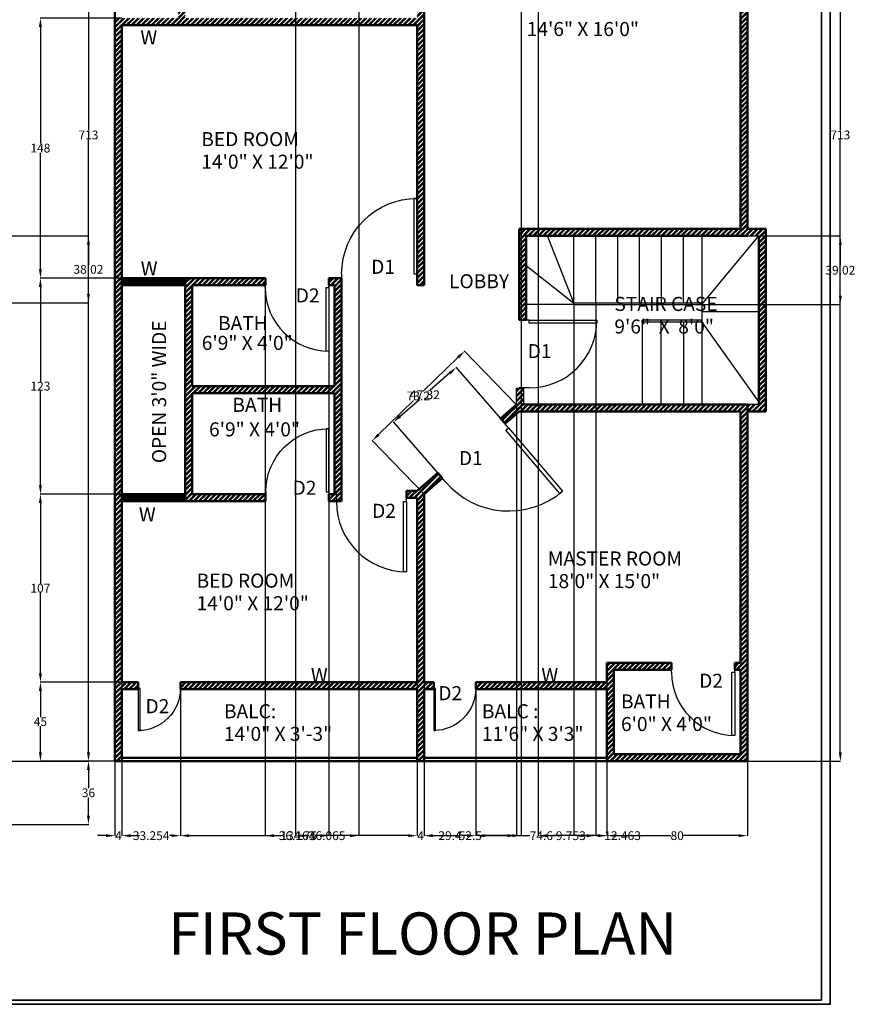
# Model space of a CAD drawing. Units: inches. Extents: x -35 to 905, y -602 to 298.
# Tile 3 of 4: x 429 to 905, y -602 to -42. Entities that reach past the tile are written whole.
import ezdxf

# ---------------------------------------------------------------- set-up
doc = ezdxf.new("R2010")
doc.units = ezdxf.units.IN
doc.header["$MEASUREMENT"] = 0
for name, color, linetype, lineweight in [('A-ANNO-DIMS', 2, 'Continuous', 18), ('A-ANNO-TEXT', 3, 'Continuous', 18), ('A-ANNO-TTLB', 7, 'Continuous', 35), ('A-AREA-IDEN', 7, 'Continuous', 18), ('A-COLS', 7, 'Continuous', 35), ('A-DOOR', 4, 'Continuous', 25), ('A-FLOR-STRS', 3, 'Continuous', 25), ('A-WALL', 7, 'Continuous', 50), ('A-WALL-PATT', 8, 'Continuous', 13)]:
    doc.layers.add(name, color=color, linetype=linetype, lineweight=lineweight)
doc.styles.get("Standard").update_dxf_attribs({"font": 'arial.ttf'})
doc.dimstyles.get("Standard").update_dxf_attribs({"dimtxt": 5, "dimasz": 5, "dimexe": 0.18, "dimexo": 0.0625, "dimgap": 0.09, "dimtad": 0, "dimtih": 1, "dimtoh": 1, "dimdec": 1, "dimzin": 0, "dimdsep": 46, "dimlunit": 4, "dimtxsty": 'Standard', "dimcen": 0.09, "dimadec": 0, "dimazin": 0, "dimtfac": 1, "dimtdec": 1, "dimtofl": 0, "dimtmove": 0, "dimatfit": 3, "dimfxl": 1, "dimtolj": 1, "dimtzin": 0, "dimarcsym": 0})

# ---------------------------------------------------------------- blocks, each defined once
blk = doc.blocks.new('*U2')
for p, q in [((0, 0), (0, -6)), ((40, 0), (40, -6))]:
    blk.add_line(p, q)
blk.add_lwpolyline([(0, 0), (0, 40), (1.75, 40), (1.75, 0)], close=True)
blk.add_arc((0, 0), 40, 0, 90)
blk = doc.blocks.new('*D17')
at = {"layer": 'A-ANNO-DIMS', "color": 0, "lineweight": -2, "ltscale": 0.3, "transparency": 16777216}
for p, q in [((377.85, -463.65), (468.36, -463.65)), ((468.18, -468.65), (468.18, -479.01)), ((468.18, -494.65), (468.18, -484.3)), ((377.85, -499.65), (468.36, -499.65))]:
    blk.add_line(p, q, dxfattribs=at)
at = {"layer": 'A-ANNO-DIMS', "color": 0, "ltscale": 0.3, "transparency": 16777216}
for points in [[(467.35, -468.65), (469.02, -468.65), (468.18, -463.65)], [(467.35, -494.65), (469.02, -494.65), (468.18, -499.65)]]:
    blk.add_solid(points, dxfattribs=at)
at = {"layer": 'Defpoints', "color": 0, "ltscale": 0.3, "transparency": 16777216}
for p in [(377.78, -463.65), (377.78, -499.65), (468.18, -499.65)]:
    blk.add_point(p, dxfattribs=at)
at = {"layer": 'A-ANNO-DIMS', "color": 0, "ltscale": 0.3, "transparency": 16777216, "insert": (468.18, -481.65), "char_height": 5, "attachment_point": 5}
blk.add_mtext('\\A1;36', dxfattribs=at)
blk = doc.blocks.new('*D18')
at = {"layer": 'A-ANNO-DIMS', "color": 0, "lineweight": -2, "ltscale": 0.3, "transparency": 16777216}
for p, q in [((377.85, 249.35), (468.36, 249.35)), ((468.18, 244.35), (468.18, -104.51)), ((468.18, -458.65), (468.18, -109.8)), ((377.85, -463.65), (468.36, -463.65))]:
    blk.add_line(p, q, dxfattribs=at)
at = {"layer": 'A-ANNO-DIMS', "color": 0, "ltscale": 0.3, "transparency": 16777216}
for points in [[(467.35, 244.35), (469.02, 244.35), (468.18, 249.35)], [(467.35, -458.65), (469.02, -458.65), (468.18, -463.65)]]:
    blk.add_solid(points, dxfattribs=at)
at = {"layer": 'Defpoints', "color": 0, "ltscale": 0.3, "transparency": 16777216}
for p in [(377.78, 249.35), (377.78, -463.65), (468.18, -463.65)]:
    blk.add_point(p, dxfattribs=at)
at = {"layer": 'A-ANNO-DIMS', "color": 0, "ltscale": 0.3, "transparency": 16777216, "insert": (468.18, -107.15), "char_height": 5, "attachment_point": 5}
blk.add_mtext('\\A1;713', dxfattribs=at)
blk = doc.blocks.new('*D28')
at = {"layer": 'A-ANNO-DIMS', "color": 0, "lineweight": -2, "ltscale": 0.3, "transparency": 16777216}
for p, q in [((279.1, -164.65), (468.36, -164.65)), ((468.18, -169.65), (468.18, -181.02)), ((468.18, -197.67), (468.18, -186.31)), ((279.1, -202.67), (468.36, -202.67))]:
    blk.add_line(p, q, dxfattribs=at)
at = {"layer": 'A-ANNO-DIMS', "color": 0, "ltscale": 0.3, "transparency": 16777216}
for points in [[(467.35, -169.65), (469.02, -169.65), (468.18, -164.65)], [(467.35, -197.67), (469.02, -197.67), (468.18, -202.67)]]:
    blk.add_solid(points, dxfattribs=at)
at = {"layer": 'Defpoints', "color": 0, "ltscale": 0.3, "transparency": 16777216}
for p in [(279.03, -164.65), (279.03, -202.67), (468.18, -202.67)]:
    blk.add_point(p, dxfattribs=at)
at = {"layer": 'A-ANNO-DIMS', "color": 0, "ltscale": 0.3, "transparency": 16777216, "insert": (468.18, -183.66), "char_height": 5, "attachment_point": 5}
blk.add_mtext('\\A1;38.02', dxfattribs=at)
blk = doc.blocks.new('*D36')
at = {"layer": 'A-ANNO-DIMS', "color": 0, "lineweight": -2, "ltscale": 0.3, "transparency": 16777216}
for p, q in [((487.18, -40.65), (440.66, -40.65)), ((440.84, -45.65), (440.84, -112.01)), ((440.84, -183.65), (440.84, -117.3)), ((487.18, -188.65), (440.66, -188.65))]:
    blk.add_line(p, q, dxfattribs=at)
at = {"layer": 'A-ANNO-DIMS', "color": 0, "ltscale": 0.3, "transparency": 16777216}
for points in [[(440.01, -45.65), (441.67, -45.65), (440.84, -40.65)], [(440.01, -183.65), (441.67, -183.65), (440.84, -188.65)]]:
    blk.add_solid(points, dxfattribs=at)
at = {"layer": 'Defpoints', "color": 0, "ltscale": 0.3, "transparency": 16777216}
for p in [(487.24, -40.65), (440.84, -188.65), (487.24, -188.65)]:
    blk.add_point(p, dxfattribs=at)
at = {"layer": 'A-ANNO-DIMS', "color": 0, "ltscale": 0.3, "transparency": 16777216, "insert": (440.84, -114.65), "char_height": 5, "attachment_point": 5}
blk.add_mtext('\\A1;148', dxfattribs=at)
blk = doc.blocks.new('*D37')
at = {"layer": 'A-ANNO-DIMS', "color": 0, "lineweight": -2, "ltscale": 0.3, "transparency": 16777216}
for p, q in [((487.18, -188.65), (440.66, -188.65)), ((440.84, -193.65), (440.84, -247.51)), ((440.84, -306.65), (440.84, -252.8)), ((487.18, -311.65), (440.66, -311.65))]:
    blk.add_line(p, q, dxfattribs=at)
at = {"layer": 'A-ANNO-DIMS', "color": 0, "ltscale": 0.3, "transparency": 16777216}
for points in [[(440.01, -193.65), (441.67, -193.65), (440.84, -188.65)], [(440.01, -306.65), (441.67, -306.65), (440.84, -311.65)]]:
    blk.add_solid(points, dxfattribs=at)
at = {"layer": 'Defpoints', "color": 0, "ltscale": 0.3, "transparency": 16777216}
for p in [(487.24, -188.65), (440.84, -311.65), (487.24, -311.65)]:
    blk.add_point(p, dxfattribs=at)
at = {"layer": 'A-ANNO-DIMS', "color": 0, "ltscale": 0.3, "transparency": 16777216, "insert": (440.84, -250.15), "char_height": 5, "attachment_point": 5}
blk.add_mtext('\\A1;123', dxfattribs=at)
blk = doc.blocks.new('*D38')
at = {"layer": 'A-ANNO-DIMS', "color": 0, "lineweight": -2, "ltscale": 0.3, "transparency": 16777216}
for p, q in [((487.18, -311.65), (440.66, -311.65)), ((440.84, -316.65), (440.84, -362.51)), ((440.84, -413.65), (440.84, -367.8)), ((487.18, -418.65), (440.66, -418.65))]:
    blk.add_line(p, q, dxfattribs=at)
at = {"layer": 'A-ANNO-DIMS', "color": 0, "ltscale": 0.3, "transparency": 16777216}
for points in [[(440.01, -316.65), (441.67, -316.65), (440.84, -311.65)], [(440.01, -413.65), (441.67, -413.65), (440.84, -418.65)]]:
    blk.add_solid(points, dxfattribs=at)
at = {"layer": 'Defpoints', "color": 0, "ltscale": 0.3, "transparency": 16777216}
for p in [(487.24, -311.65), (440.84, -418.65), (487.24, -418.65)]:
    blk.add_point(p, dxfattribs=at)
at = {"layer": 'A-ANNO-DIMS', "color": 0, "ltscale": 0.3, "transparency": 16777216, "insert": (440.84, -365.15), "char_height": 5, "attachment_point": 5}
blk.add_mtext('\\A1;107', dxfattribs=at)
blk = doc.blocks.new('*D39')
at = {"layer": 'A-ANNO-DIMS', "color": 0, "lineweight": -2, "ltscale": 0.3, "transparency": 16777216}
for p, q in [((487.18, -418.65), (440.66, -418.65)), ((440.84, -423.65), (440.84, -438.52)), ((440.84, -458.65), (440.84, -443.79)), ((483.18, -463.65), (440.66, -463.65))]:
    blk.add_line(p, q, dxfattribs=at)
at = {"layer": 'A-ANNO-DIMS', "color": 0, "ltscale": 0.3, "transparency": 16777216}
for points in [[(440.01, -423.65), (441.67, -423.65), (440.84, -418.65)], [(440.01, -458.65), (441.67, -458.65), (440.84, -463.65)]]:
    blk.add_solid(points, dxfattribs=at)
at = {"layer": 'Defpoints', "color": 0, "ltscale": 0.3, "transparency": 16777216}
for p in [(487.24, -418.65), (440.84, -463.65), (483.24, -463.65)]:
    blk.add_point(p, dxfattribs=at)
at = {"layer": 'A-ANNO-DIMS', "color": 0, "ltscale": 0.3, "transparency": 16777216, "insert": (440.84, -441.15), "char_height": 5, "attachment_point": 5}
blk.add_mtext('\\A1;45', dxfattribs=at)
blk = doc.blocks.new('*D40')
at = {"layer": 'A-ANNO-DIMS', "color": 0, "lineweight": -2, "ltscale": 0.3, "transparency": 16777216}
for p, q in [((843.3, 249.35), (896.28, 249.35)), ((896.1, 244.35), (896.1, -104.51)), ((896.1, -458.65), (896.1, -109.8)), ((843.3, -463.65), (896.28, -463.65))]:
    blk.add_line(p, q, dxfattribs=at)
at = {"layer": 'A-ANNO-DIMS', "color": 0, "ltscale": 0.3, "transparency": 16777216}
for points in [[(895.27, 244.35), (896.94, 244.35), (896.1, 249.35)], [(895.27, -458.65), (896.94, -458.65), (896.1, -463.65)]]:
    blk.add_solid(points, dxfattribs=at)
at = {"layer": 'Defpoints', "color": 0, "ltscale": 0.3, "transparency": 16777216}
for p in [(843.24, 249.35), (843.24, -463.65), (896.1, -463.65)]:
    blk.add_point(p, dxfattribs=at)
at = {"layer": 'A-ANNO-DIMS', "color": 0, "ltscale": 0.3, "transparency": 16777216, "insert": (896.1, -107.15), "char_height": 5, "attachment_point": 5}
blk.add_mtext('\\A1;713', dxfattribs=at)
blk = doc.blocks.new('*D41')
at = {"layer": 'A-ANNO-DIMS', "color": 0, "lineweight": -2, "ltscale": 0.3, "transparency": 16777216}
for p, q in [((487.24, -418.72), (487.24, -506.23)), ((483.24, -463.72), (483.24, -506.23)), ((478.24, -506.05), (473.24, -506.05)), ((492.24, -506.05), (497.24, -506.05))]:
    blk.add_line(p, q, dxfattribs=at)
at = {"layer": 'A-ANNO-DIMS', "color": 0, "ltscale": 0.3, "transparency": 16777216}
for points in [[(478.24, -505.22), (478.24, -506.89), (483.24, -506.05)], [(492.24, -505.22), (492.24, -506.89), (487.24, -506.05)]]:
    blk.add_solid(points, dxfattribs=at)
at = {"layer": 'Defpoints', "color": 0, "ltscale": 0.3, "transparency": 16777216}
for p in [(487.24, -418.65), (483.24, -463.65), (487.24, -506.05)]:
    blk.add_point(p, dxfattribs=at)
at = {"layer": 'A-ANNO-DIMS', "color": 0, "ltscale": 0.3, "transparency": 16777216, "insert": (485.24, -506.05), "char_height": 5, "attachment_point": 5}
blk.add_mtext('\\A1;4', dxfattribs=at)
blk = doc.blocks.new('*D42')
at = {"layer": 'A-ANNO-DIMS', "color": 0, "lineweight": -2, "ltscale": 0.3, "transparency": 16777216}
for p, q in [((487.24, -418.72), (487.24, -506.23)), ((520.49, -418.72), (520.49, -506.23)), ((492.24, -506.05), (493.41, -506.05)), ((515.49, -506.05), (514.32, -506.05))]:
    blk.add_line(p, q, dxfattribs=at)
at = {"layer": 'A-ANNO-DIMS', "color": 0, "ltscale": 0.3, "transparency": 16777216}
for points in [[(492.24, -505.22), (492.24, -506.89), (487.24, -506.05)], [(515.49, -505.22), (515.49, -506.89), (520.49, -506.05)]]:
    blk.add_solid(points, dxfattribs=at)
at = {"layer": 'Defpoints', "color": 0, "ltscale": 0.3, "transparency": 16777216}
for p in [(487.24, -418.65), (520.49, -418.65), (520.49, -506.05)]:
    blk.add_point(p, dxfattribs=at)
at = {"layer": 'A-ANNO-DIMS', "color": 0, "ltscale": 0.3, "transparency": 16777216, "insert": (503.87, -506.05), "char_height": 5, "attachment_point": 5}
blk.add_mtext('\\A1;33.254', dxfattribs=at)
blk = doc.blocks.new('*D43')
at = {"layer": 'A-ANNO-DIMS', "color": 0, "lineweight": -2, "ltscale": 0.3, "transparency": 16777216}
for p, q in [((520.49, -418.72), (520.49, -506.23)), ((655.24, -418.72), (655.24, -506.23)), ((525.49, -506.05), (577.61, -506.05)), ((650.24, -506.05), (598.12, -506.05))]:
    blk.add_line(p, q, dxfattribs=at)
at = {"layer": 'A-ANNO-DIMS', "color": 0, "ltscale": 0.3, "transparency": 16777216}
for points in [[(525.49, -505.22), (525.49, -506.89), (520.49, -506.05)], [(650.24, -505.22), (650.24, -506.89), (655.24, -506.05)]]:
    blk.add_solid(points, dxfattribs=at)
at = {"layer": 'Defpoints', "color": 0, "ltscale": 0.3, "transparency": 16777216}
for p in [(520.49, -418.65), (655.24, -418.65), (655.24, -506.05)]:
    blk.add_point(p, dxfattribs=at)
at = {"layer": 'A-ANNO-DIMS', "color": 0, "ltscale": 0.3, "transparency": 16777216, "insert": (587.87, -506.05), "char_height": 5, "attachment_point": 5}
blk.add_mtext('\\A1;134.75', dxfattribs=at)
blk = doc.blocks.new('*D44')
at = {"layer": 'A-ANNO-DIMS', "color": 0, "lineweight": -2, "ltscale": 0.3, "transparency": 16777216}
for p, q in [((655.24, -418.72), (655.24, -506.23)), ((659.24, -418.72), (659.24, -506.23)), ((650.24, -506.05), (645.24, -506.05)), ((664.24, -506.05), (669.24, -506.05))]:
    blk.add_line(p, q, dxfattribs=at)
at = {"layer": 'A-ANNO-DIMS', "color": 0, "ltscale": 0.3, "transparency": 16777216}
for points in [[(650.24, -505.22), (650.24, -506.89), (655.24, -506.05)], [(664.24, -505.22), (664.24, -506.89), (659.24, -506.05)]]:
    blk.add_solid(points, dxfattribs=at)
at = {"layer": 'Defpoints', "color": 0, "ltscale": 0.3, "transparency": 16777216}
for p in [(655.24, -418.65), (659.24, -418.65), (659.24, -506.05)]:
    blk.add_point(p, dxfattribs=at)
at = {"layer": 'A-ANNO-DIMS', "color": 0, "ltscale": 0.3, "transparency": 16777216, "insert": (657.24, -506.05), "char_height": 5, "attachment_point": 5}
blk.add_mtext('\\A1;4', dxfattribs=at)
blk = doc.blocks.new('*D45')
at = {"layer": 'A-ANNO-DIMS', "color": 0, "lineweight": -2, "ltscale": 0.3, "transparency": 16777216}
for p, q in [((659.24, -418.72), (659.24, -506.23)), ((688.64, -418.72), (688.64, -506.23)), ((664.24, -506.05), (667.32, -506.05)), ((683.64, -506.05), (680.55, -506.05))]:
    blk.add_line(p, q, dxfattribs=at)
at = {"layer": 'A-ANNO-DIMS', "color": 0, "ltscale": 0.3, "transparency": 16777216}
for points in [[(664.24, -505.22), (664.24, -506.89), (659.24, -506.05)], [(683.64, -505.22), (683.64, -506.89), (688.64, -506.05)]]:
    blk.add_solid(points, dxfattribs=at)
at = {"layer": 'Defpoints', "color": 0, "ltscale": 0.3, "transparency": 16777216}
for p in [(659.24, -418.65), (688.64, -418.65), (688.64, -506.05)]:
    blk.add_point(p, dxfattribs=at)
at = {"layer": 'A-ANNO-DIMS', "color": 0, "ltscale": 0.3, "transparency": 16777216, "insert": (673.94, -506.05), "char_height": 5, "attachment_point": 5}
blk.add_mtext('\\A1;29.4', dxfattribs=at)
blk = doc.blocks.new('*D46')
at = {"layer": 'A-ANNO-DIMS', "color": 0, "lineweight": -2, "ltscale": 0.3, "transparency": 16777216}
for p, q in [((688.64, -418.72), (688.64, -506.23)), ((763.24, -418.72), (763.24, -506.23)), ((693.64, -506.05), (719.38, -506.05)), ((758.24, -506.05), (732.5, -506.05))]:
    blk.add_line(p, q, dxfattribs=at)
at = {"layer": 'A-ANNO-DIMS', "color": 0, "ltscale": 0.3, "transparency": 16777216}
for points in [[(693.64, -505.22), (693.64, -506.89), (688.64, -506.05)], [(758.24, -505.22), (758.24, -506.89), (763.24, -506.05)]]:
    blk.add_solid(points, dxfattribs=at)
at = {"layer": 'Defpoints', "color": 0, "ltscale": 0.3, "transparency": 16777216}
for p in [(688.64, -418.65), (763.24, -418.65), (763.24, -506.05)]:
    blk.add_point(p, dxfattribs=at)
at = {"layer": 'A-ANNO-DIMS', "color": 0, "ltscale": 0.3, "transparency": 16777216, "insert": (725.94, -506.05), "char_height": 5, "attachment_point": 5}
blk.add_mtext('\\A1;74.6', dxfattribs=at)
blk = doc.blocks.new('*D47')
at = {"layer": 'A-ANNO-DIMS', "color": 0, "lineweight": -2, "ltscale": 0.3, "transparency": 16777216}
for p, q in [((763.24, -418.72), (763.24, -506.23)), ((843.24, -463.72), (843.24, -506.23)), ((768.24, -506.05), (799.57, -506.05)), ((838.24, -506.05), (806.9, -506.05))]:
    blk.add_line(p, q, dxfattribs=at)
at = {"layer": 'A-ANNO-DIMS', "color": 0, "ltscale": 0.3, "transparency": 16777216}
for points in [[(768.24, -505.22), (768.24, -506.89), (763.24, -506.05)], [(838.24, -505.22), (838.24, -506.89), (843.24, -506.05)]]:
    blk.add_solid(points, dxfattribs=at)
at = {"layer": 'Defpoints', "color": 0, "ltscale": 0.3, "transparency": 16777216}
for p in [(763.24, -418.65), (843.24, -463.65), (843.24, -506.05)]:
    blk.add_point(p, dxfattribs=at)
at = {"layer": 'A-ANNO-DIMS', "color": 0, "ltscale": 0.3, "transparency": 16777216, "insert": (803.24, -506.05), "char_height": 5, "attachment_point": 5}
blk.add_mtext('\\A1;80', dxfattribs=at)
blk = doc.blocks.new('*D48')
at = {"layer": 'A-ANNO-DIMS', "color": 0, "lineweight": -2, "ltscale": 0.3, "transparency": 16777216}
for p, q in [((585.99, 167.28), (585.99, -506.23)), ((622.06, 167.28), (622.06, -506.23)), ((590.99, -506.05), (593.54, -506.05)), ((617.06, -506.05), (614.51, -506.05))]:
    blk.add_line(p, q, dxfattribs=at)
at = {"layer": 'A-ANNO-DIMS', "color": 0, "ltscale": 0.3, "transparency": 16777216}
for points in [[(590.99, -505.22), (590.99, -506.89), (585.99, -506.05)], [(617.06, -505.22), (617.06, -506.89), (622.06, -506.05)]]:
    blk.add_solid(points, dxfattribs=at)
at = {"layer": 'Defpoints', "color": 0, "ltscale": 0.3, "transparency": 16777216}
for p in [(585.99, 167.35), (622.06, 167.35), (622.06, -506.05)]:
    blk.add_point(p, dxfattribs=at)
at = {"layer": 'A-ANNO-DIMS', "color": 0, "ltscale": 0.3, "transparency": 16777216, "insert": (604.02, -506.05), "char_height": 5, "attachment_point": 5}
blk.add_mtext('\\A1;36.065', dxfattribs=at)
blk = doc.blocks.new('*D49')
at = {"layer": 'A-ANNO-DIMS', "color": 0, "lineweight": -2, "ltscale": 0.3, "transparency": 16777216}
for p, q in [((568.83, -188.72), (568.83, -506.23)), ((604.99, -188.72), (604.99, -506.23)), ((573.83, -506.05), (576.45, -506.05)), ((599.99, -506.05), (597.37, -506.05))]:
    blk.add_line(p, q, dxfattribs=at)
at = {"layer": 'A-ANNO-DIMS', "color": 0, "ltscale": 0.3, "transparency": 16777216}
for points in [[(573.83, -505.22), (573.83, -506.89), (568.83, -506.05)], [(599.99, -505.22), (599.99, -506.89), (604.99, -506.05)]]:
    blk.add_solid(points, dxfattribs=at)
at = {"layer": 'Defpoints', "color": 0, "ltscale": 0.3, "transparency": 16777216}
for p in [(568.83, -188.65), (604.99, -188.65), (604.99, -506.05)]:
    blk.add_point(p, dxfattribs=at)
at = {"layer": 'A-ANNO-DIMS', "color": 0, "ltscale": 0.3, "transparency": 16777216, "insert": (586.91, -506.05), "char_height": 5, "attachment_point": 5}
blk.add_mtext('\\A1;36.164', dxfattribs=at)
blk = doc.blocks.new('*D50')
at = {"layer": 'A-ANNO-DIMS', "color": 0, "lineweight": -2, "ltscale": 0.3, "transparency": 16777216}
for p, q in [((705.33, -271.45), (677.42, -239.38)), ((673.76, -242.8), (662.73, -252.41)), ((645.62, -267.3), (656.65, -257.7)), ((669.64, -302.52), (641.73, -270.45))]:
    blk.add_line(p, q, dxfattribs=at)
at = {"layer": 'A-ANNO-DIMS', "color": 0, "ltscale": 0.3, "transparency": 16777216}
for points in [[(673.22, -242.17), (674.31, -243.43), (677.53, -239.52)], [(645.07, -266.67), (646.16, -267.93), (641.84, -270.58)]]:
    blk.add_solid(points, dxfattribs=at)
at = {"layer": 'Defpoints', "color": 0, "ltscale": 0.3, "transparency": 16777216}
for p in [(677.53, -239.52), (705.37, -271.5), (669.68, -302.57)]:
    blk.add_point(p, dxfattribs=at)
at = {"layer": 'A-ANNO-DIMS', "color": 0, "ltscale": 0.3, "transparency": 16777216, "insert": (659.69, -255.05), "char_height": 5, "attachment_point": 5}
blk.add_mtext('\\A1;47.32', dxfattribs=at)
blk = doc.blocks.new('*D52')
at = {"layer": 'A-ANNO-DIMS', "color": 0, "lineweight": -2, "ltscale": 0.3, "transparency": 16777216}
for p, q in [((714.42, 202.86), (714.42, -506.23)), ((724.17, 202.86), (724.17, -506.23)), ((709.42, -506.05), (704.42, -506.05)), ((729.17, -506.05), (734.17, -506.05))]:
    blk.add_line(p, q, dxfattribs=at)
at = {"layer": 'A-ANNO-DIMS', "color": 0, "ltscale": 0.3, "transparency": 16777216}
for points in [[(709.42, -505.22), (709.42, -506.89), (714.42, -506.05)], [(729.17, -505.22), (729.17, -506.89), (724.17, -506.05)]]:
    blk.add_solid(points, dxfattribs=at)
at = {"layer": 'Defpoints', "color": 0, "ltscale": 0.3, "transparency": 16777216}
for p in [(714.42, 202.92), (724.17, 202.92), (724.17, -506.05)]:
    blk.add_point(p, dxfattribs=at)
at = {"layer": 'A-ANNO-DIMS', "color": 0, "ltscale": 0.3, "transparency": 16777216, "insert": (742.7, -506.05), "char_height": 5, "attachment_point": 5}
blk.add_mtext('\\A1;9.753', dxfattribs=at)
blk = doc.blocks.new('*D54')
at = {"layer": 'A-ANNO-DIMS', "color": 0, "lineweight": -2, "ltscale": 0.3, "transparency": 16777216}
for p, q in [((744.49, -203.74), (744.49, -506.23)), ((756.95, -202.74), (756.95, -506.23)), ((749.49, -506.05), (751.95, -506.05)), ((756.95, -506.05), (761.95, -506.05))]:
    blk.add_line(p, q, dxfattribs=at)
at = {"layer": 'A-ANNO-DIMS', "color": 0, "ltscale": 0.3, "transparency": 16777216}
for points in [[(749.49, -505.22), (749.49, -506.89), (744.49, -506.05)], [(751.95, -505.22), (751.95, -506.89), (756.95, -506.05)]]:
    blk.add_solid(points, dxfattribs=at)
at = {"layer": 'Defpoints', "color": 0, "ltscale": 0.3, "transparency": 16777216}
for p in [(744.49, -203.67), (756.95, -202.67), (756.95, -506.05)]:
    blk.add_point(p, dxfattribs=at)
at = {"layer": 'A-ANNO-DIMS', "color": 0, "ltscale": 0.3, "transparency": 16777216, "insert": (772.18, -506.05), "char_height": 5, "attachment_point": 5}
blk.add_mtext('\\A1;12.463', dxfattribs=at)
blk = doc.blocks.new('*D55')
at = {"layer": 'A-ANNO-DIMS', "color": 0, "lineweight": -2, "ltscale": 0.3, "transparency": 16777216}
for p, q in [((744.55, -164.65), (896.28, -164.65)), ((896.1, -169.65), (896.1, -181.52)), ((896.1, -198.67), (896.1, -186.81)), ((744.55, -203.67), (896.28, -203.67))]:
    blk.add_line(p, q, dxfattribs=at)
at = {"layer": 'A-ANNO-DIMS', "color": 0, "ltscale": 0.3, "transparency": 16777216}
for points in [[(895.27, -169.65), (896.94, -169.65), (896.1, -164.65)], [(895.27, -198.67), (896.94, -198.67), (896.1, -203.67)]]:
    blk.add_solid(points, dxfattribs=at)
at = {"layer": 'Defpoints', "color": 0, "ltscale": 0.3, "transparency": 16777216}
for p in [(744.49, -164.65), (744.49, -203.67), (896.1, -203.67)]:
    blk.add_point(p, dxfattribs=at)
at = {"layer": 'A-ANNO-DIMS', "color": 0, "ltscale": 0.3, "transparency": 16777216, "insert": (896.1, -184.16), "char_height": 5, "attachment_point": 5}
blk.add_mtext('\\A1;39.02', dxfattribs=at)
blk = doc.blocks.new('*D56')
at = {"layer": 'A-ANNO-DIMS', "color": 0, "lineweight": -2, "ltscale": 0.3, "transparency": 16777216}
for p, q in [((711.74, -260.72), (711.74, -506.23)), ((659.24, -311.72), (659.24, -506.23)), ((664.24, -506.05), (678.89, -506.05)), ((706.74, -506.05), (692.09, -506.05))]:
    blk.add_line(p, q, dxfattribs=at)
at = {"layer": 'A-ANNO-DIMS', "color": 0, "ltscale": 0.3, "transparency": 16777216}
for points in [[(664.24, -505.22), (664.24, -506.89), (659.24, -506.05)], [(706.74, -505.22), (706.74, -506.89), (711.74, -506.05)]]:
    blk.add_solid(points, dxfattribs=at)
at = {"layer": 'Defpoints', "color": 0, "ltscale": 0.3, "transparency": 16777216}
for p in [(711.74, -260.65), (659.24, -311.65), (711.74, -506.05)]:
    blk.add_point(p, dxfattribs=at)
at = {"layer": 'A-ANNO-DIMS', "color": 0, "ltscale": 0.3, "transparency": 16777216, "insert": (685.49, -506.05), "char_height": 5, "attachment_point": 5}
blk.add_mtext('\\A1;52.5', dxfattribs=at)
blk = doc.blocks.new('*D57')
at = {"layer": 'A-ANNO-DIMS', "color": 0, "lineweight": -2, "ltscale": 0.3, "transparency": 16777216}
for p, q in [((678.61, -233.72), (658.67, -253.1)), ((711.7, -260.61), (682.07, -230.11)), ((633.28, -277.76), (653.22, -258.38)), ((659.19, -311.61), (629.57, -281.11))]:
    blk.add_line(p, q, dxfattribs=at)
at = {"layer": 'A-ANNO-DIMS', "color": 0, "ltscale": 0.3, "transparency": 16777216}
for points in [[(678.03, -233.13), (679.19, -234.32), (682.2, -230.24)], [(632.7, -277.16), (633.86, -278.35), (629.7, -281.24)]]:
    blk.add_solid(points, dxfattribs=at)
at = {"layer": 'Defpoints', "color": 0, "ltscale": 0.3, "transparency": 16777216}
for p in [(682.2, -230.24), (711.74, -260.65), (659.24, -311.65)]:
    blk.add_point(p, dxfattribs=at)
at = {"layer": 'A-ANNO-DIMS', "color": 0, "ltscale": 0.3, "transparency": 16777216, "insert": (655.95, -255.74), "char_height": 5, "attachment_point": 5}
blk.add_mtext('\\A1;73.2', dxfattribs=at)

msp = doc.modelspace()

# ---------------------------------------------------------------- hatches: boundary and pattern name
at = {"layer": 'A-WALL-PATT', "ltscale": 0.3}
h = msp.add_hatch(dxfattribs=at)
h.set_pattern_fill('ANSI32', color=256, scale=5.3)
h.set_pattern_definition([(45, (-58.8752, 0), (-1.4053747, 1.4053747), []), (45, (-57.9383, 0), (-1.4053747, 1.4053747), [])])
h.paths.add_polyline_path([(843.2385, 107.3466), (843.2385, 249.3466), (521.2385, 249.3466), (521.2385, 171.3466), (487.2385, 171.3466), (487.2385, 167.3466), (586.0557, 167.3466), (586.0557, 171.3466), (567.2385, 171.3466), (525.2385, 171.3466), (525.2385, 243.3466), (571.2385, 243.3466), (655.2385, 243.3466), (655.2385, 213.7106), (655.2385, 171.3466), (622.0557, 171.3466), (622.0557, 167.3466), (655.2385, 167.3466), (655.2385, 79.3466), (659.2385, 79.3466), (659.2385, 107.3466), (665.2408, 107.3466), (665.2408, 111.3466), (659.2385, 111.3466), (659.2385, 213.7106), (659.2385, 243.3466), (841.2385, 243.3466), (841.2385, 111.3466), (721.2578, 111.3466), (721.2578, 107.1453), (721.2578, 81.4115), (725.2385, 81.4115), (725.2385, 107.3466), (839.2385, 107.3466), (839.2385, 35.3466), (721.2385, 35.3466), (721.2385, 31.3466), (839.2385, 31.3466), (839.2385, -160.6534), (713.2385, -160.6534), (713.2385, -164.6534), (713.2385, -212.6534), (717.2385, -212.6534), (717.2385, -164.6534), (843.2385, -164.6534), (849.7023, -164.6534), (849.7023, -260.6534), (843.2385, -260.6534), (843.2385, -264.6534), (853.7023, -264.6534), (853.7023, -160.6534), (843.2385, -160.6534)])
h.paths.add_polyline_path([(655.2385, -188.6534), (655.2385, -192.6534), (659.2385, -192.6534), (659.2385, -23.1851), (655.2385, -23.1851), (655.2385, -40.6534), (523.2385, -40.6534), (523.2385, 19.3466), (655.2385, 19.3466), (655.2385, 12.8149), (659.2385, 12.8149), (659.2385, 31.3466), (655.2385, 31.3466), (655.2385, 23.3466), (487.2385, 23.3466), (487.2385, 167.3466), (483.2385, 167.3466), (483.2385, 19.3466), (519.2385, 19.3466), (519.2385, -40.6534), (483.2385, -40.6534), (483.2385, -463.6534), (487.2385, -463.6534), (487.2385, -422.6534), (496.4926, -422.6534), (496.4926, -422.2505), (496.4926, -418.6534), (487.2385, -418.6534), (487.2385, -315.6534), (487.2385, -192.6534), (487.2385, -44.6534), (655.2385, -44.6534)])
h.paths.add_polyline_path([(523.2385, -315.6534), (568.9907, -315.6534), (568.9907, -311.6534), (527.2385, -311.6534), (527.2385, -254.1534), (608.2385, -254.1534), (608.2385, -311.6534), (604.9907, -311.6534), (604.9907, -315.6534), (612.2385, -315.6534), (612.2385, -250.1534), (612.2385, -188.6534), (604.9907, -188.6534), (604.9907, -192.6534), (608.2385, -192.6534), (608.2385, -250.1534), (527.2385, -250.1534), (527.2385, -192.6534), (568.8266, -192.6534), (568.8266, -188.6534), (523.2385, -188.6534)], flags=17)
h.paths.add_polyline_path([(655.2385, -313.832), (655.2385, -418.6534), (520.4926, -418.6534), (520.4926, -422.6534), (655.2385, -422.6534), (655.2385, -461.6534), (655.2385, -463.6534), (659.2385, -463.6534), (659.2385, -457.6052), (659.2385, -422.6534), (664.6743, -422.6534), (664.6743, -422.2478), (664.6743, -418.6534), (659.2385, -418.6534), (659.2385, -311.6534), (669.6291, -302.6097), (667.0409, -299.5595), (655.2385, -309.832), (649.2787, -309.832), (649.2787, -313.832)])
h.paths.add_polyline_path([(839.2385, -264.6534), (839.2385, -407.6534), (836.0142, -407.6534), (836.0142, -411.6534), (839.2385, -411.6534), (839.2385, -459.6534), (767.2385, -459.6534), (767.2385, -411.6534), (800.0142, -411.6534), (800.0142, -407.6534), (767.2385, -407.6534), (763.2385, -407.6534), (763.2385, -418.6534), (688.6743, -418.6534), (688.6743, -422.6534), (763.2385, -422.6534), (763.2385, -463.6534), (843.2385, -463.6534), (843.2385, -260.6534), (715.7415, -260.6534), (715.7415, -251.2468), (711.7415, -251.2468), (711.7415, -260.6534), (704.4179, -267.0277), (702.7449, -268.4838), (705.371, -271.5011), (707.044, -270.0449), (713.2385, -264.6534)])
h.paths.add_polyline_path([(592.7587, -420.6534), (607.3071, -420.6534), (607.3071, -408.6534), (592.7587, -408.6534)], flags=24)
h.paths.add_polyline_path([(723.9564, -420.6534), (738.5048, -420.6534), (738.5048, -408.6534), (723.9564, -408.6534)], flags=24)

# ---------------------------------------------------------------- linework, layer by layer
at = {"layer": 'A-ANNO-TTLB', "ltscale": 0.3}
for points in [[(-16.7606, 298.2205), (890.3824, 298.2205), (890.3824, -602.0527), (-16.7606, -602.0527)], [(-11.7606, 293.2205), (885.3824, 293.2205), (885.3824, -599.6301), (-11.7606, -599.6301)]]:
    msp.add_lwpolyline(points, close=True, dxfattribs=at)
at = {"layer": 'A-COLS'}
for points in [[(659.2385, -457.6052), (659.2385, -463.6534), (667.2239, -463.6534)], [(695.2592, -463.6534), (703.2446, -463.6534)]]:
    msp.add_lwpolyline(points, dxfattribs=at)
at = {"layer": 'A-FLOR-STRS', "ltscale": 0.3}
for p, q in [((744.4872, -202.6738), (729.4957, -164.6534)), ((744.4872, -202.6738), (744.4872, -164.6534)), ((756.9506, -202.6738), (756.9506, -164.6534)), ((769.414, -202.6738), (769.414, -164.6534)), ((781.8774, -202.6738), (781.8774, -164.6534)), ((794.3408, -202.6738), (794.3408, -164.6534)), ((806.8042, -202.6738), (806.8042, -164.6534)), ((806.8042, -202.6738), (806.8042, -164.6534)), ((817.267, -164.6534), (817.267, -202.6738)), ((817.267, -203.6738), (849.7023, -164.6534)), ((843.2385, -164.6534), (849.7023, -164.6534)), ((744.4872, -203.1738), (717.2385, -181.6178)), ((744.4872, -203.6738), (717.2385, -203.6738)), ((744.4872, -202.6738), (817.267, -202.6738)), ((744.4872, -203.6738), (744.4872, -202.6738)), ((744.4872, -203.6738), (817.267, -203.6738)), ((817.267, -202.6738), (817.267, -212.6534)), ((817.267, -212.6534), (783.2385, -212.6534)), ((783.2385, -213.6534), (783.2385, -212.6534)), ((817.267, -207.6636), (849.7023, -207.6636)), ((817.267, -212.6534), (817.267, -212.6534)), ((817.267, -212.6534), (817.267, -213.6534)), ((817.267, -213.6534), (783.2385, -213.6534)), ((783.2385, -213.6534), (783.2385, -260.6534)), ((793.8628, -213.6534), (793.8628, -260.6534)), ((806.8042, -213.6534), (806.8042, -260.6534)), ((817.267, -213.6534), (817.267, -260.6534)), ((817.267, -213.6534), (849.7023, -259.1945)), ((711.7415, -260.6534), (711.7415, -251.2468)), ((711.7415, -251.2468), (715.7415, -251.2468)), ((715.7415, -251.2468), (715.7415, -260.6534)), ((849.7023, -260.6534), (843.2385, -260.6534))]:
    msp.add_line(p, q, dxfattribs=at)
at = {"layer": 'A-FLOR-STRS'}
msp.add_line((713.2385, -212.6534), (717.2385, -212.6534), dxfattribs=at)
at = {"layer": 'A-WALL'}
for p, q in [((483.2385, 249.3466), (483.2385, -463.6534)), ((843.2385, 107.3466), (843.2385, -160.6534)), ((839.2385, 31.3466), (839.2385, -160.6534)), ((659.2385, -23.1851), (659.2385, -192.6534)), ((487.2385, -44.6534), (487.2385, -192.6534)), ((487.2385, -44.6534), (655.2385, -44.6534)), ((655.2385, -44.6534), (655.2385, -188.6534)), ((713.2385, -160.6534), (839.2385, -160.6534)), ((713.2385, -160.6534), (713.2385, -164.6534)), ((713.2385, -164.6534), (713.2385, -212.6534)), ((717.2385, -164.6534), (843.2385, -164.6534)), ((717.2385, -212.6534), (717.2385, -164.6534)), ((487.2385, -188.6534), (568.9907, -188.6534)), ((487.2385, -189.6051), (523.2385, -189.6051)), ((523.2385, -188.6534), (523.2385, -315.6534)), ((568.9907, -188.6534), (568.9907, -192.6534)), ((604.9907, -188.6534), (612.2385, -188.6534)), ((604.9907, -192.6534), (604.9907, -188.6534)), ((612.2385, -188.6534), (612.2385, -250.1534)), ((655.2385, -188.6534), (655.2385, -192.6534)), ((487.2385, -190.8554), (523.2385, -190.8554)), ((487.2385, -191.7877), (523.2385, -191.7877)), ((487.2385, -192.6534), (487.2385, -315.6534)), ((487.2385, -192.6534), (523.2385, -192.6534)), ((527.2385, -192.6534), (527.2385, -250.1534)), ((527.2385, -192.6534), (568.9907, -192.6534)), ((604.9907, -192.6534), (608.2385, -192.6534)), ((608.2385, -192.6534), (608.2385, -250.1534)), ((655.2385, -192.6534), (659.2385, -192.6534)), ((527.2385, -250.1534), (608.2385, -250.1534)), ((612.2385, -250.1534), (612.2385, -315.6534)), ((527.2385, -254.1534), (527.2385, -311.6534)), ((527.2385, -254.1534), (608.2385, -254.1534)), ((608.2385, -254.1534), (608.2385, -311.6534)), ((704.4179, -267.0277), (711.7415, -260.6534)), ((715.7415, -260.6534), (843.2385, -260.6534)), ((843.2385, -260.6534), (843.2385, -463.6534)), ((702.7449, -268.4838), (704.4179, -267.0277)), ((707.044, -270.0449), (713.2385, -264.6534)), ((713.2385, -264.6534), (839.2385, -264.6534)), ((839.2385, -264.6534), (839.2385, -407.6534)), ((705.371, -271.5011), (707.044, -270.0449)), ((655.2385, -309.832), (667.0543, -299.5479)), ((659.2385, -311.6534), (669.6804, -302.5651)), ((487.2385, -311.6534), (523.2385, -311.6534)), ((487.2385, -312.3877), (523.2385, -312.3877)), ((487.2385, -313.638), (523.2385, -313.638)), ((527.2385, -311.6534), (568.9907, -311.6534)), ((568.9907, -311.6534), (568.9907, -315.6534)), ((604.9907, -311.6534), (608.2385, -311.6534)), ((604.9907, -315.6534), (604.9907, -311.6534)), ((655.2385, -313.832), (655.2385, -315.6534)), ((655.2385, -313.832), (655.2385, -418.6534)), ((659.2385, -311.6534), (659.2385, -418.6534)), ((487.2385, -314.5703), (523.2385, -314.5703)), ((487.2385, -315.6534), (487.2385, -418.6534)), ((487.2385, -315.6534), (568.9907, -315.6534)), ((604.9907, -315.6534), (612.2385, -315.6534)), ((767.2385, -407.6534), (800.0142, -407.6534)), ((836.0142, -407.6534), (839.2385, -407.6534)), ((767.2385, -411.6534), (767.2385, -459.6534)), ((767.2385, -411.6534), (800.0142, -411.6534)), ((836.0142, -411.6534), (839.2385, -411.6534)), ((839.2385, -411.6534), (839.2385, -459.6534)), ((487.2385, -418.6534), (496.4926, -418.6534)), ((520.4926, -418.6534), (655.2385, -418.6534)), ((659.2385, -418.6534), (664.6743, -418.6534)), ((688.6743, -418.6534), (763.2385, -418.6534)), ((487.2385, -422.6534), (496.4926, -422.6534)), ((487.2385, -422.6534), (487.2385, -463.6534)), ((520.4926, -422.6534), (655.2385, -422.6534)), ((655.2385, -422.6534), (655.2385, -461.6534)), ((659.2385, -422.6534), (664.6743, -422.6534)), ((659.2385, -422.6534), (659.2385, -461.6534)), ((688.6743, -422.6534), (763.2385, -422.6534)), ((763.2385, -422.6534), (763.2385, -463.6534)), ((483.2385, -463.6534), (487.2385, -463.6534)), ((487.2385, -461.6534), (655.2385, -461.6534)), ((487.2385, -463.6534), (655.2385, -463.6534)), ((655.2385, -461.6534), (655.2385, -463.6534)), ((655.2385, -463.6534), (763.2385, -463.6534)), ((659.2385, -461.6534), (695.2592, -461.6534)), ((659.2385, -461.6534), (659.2385, -463.6534)), ((695.2592, -461.6534), (763.2385, -461.6534)), ((763.2385, -463.6534), (843.2385, -463.6534)), ((767.2385, -459.6534), (839.2385, -459.6534))]:
    msp.add_line(p, q, dxfattribs=at)
at = {"layer": 'A-WALL', "ltscale": 0.3}
for p, q in [((843.2385, -160.6534), (853.7023, -160.6534)), ((853.7023, -160.6534), (853.7023, -264.6534)), ((849.7023, -164.6534), (849.7023, -260.6534)), ((705.371, -271.5011), (702.7449, -268.4838)), ((853.7023, -264.6534), (843.2385, -264.6534)), ((667.0543, -299.5479), (669.6804, -302.5651)), ((655.2385, -309.832), (649.2787, -309.832)), ((649.2787, -309.832), (649.2787, -313.832)), ((649.2787, -313.832), (655.2385, -313.832)), ((767.2385, -407.6534), (763.2385, -407.6534)), ((763.2385, -407.6534), (763.2385, -418.6534)), ((800.0142, -407.6534), (800.0142, -411.6534)), ((836.0142, -411.6534), (836.0142, -407.6534)), ((496.4926, -418.6534), (496.4926, -422.6534)), ((520.4926, -418.6534), (520.4926, -422.6534)), ((664.6743, -418.6534), (664.6743, -422.6534)), ((688.6743, -422.6534), (688.6743, -418.6534))]:
    msp.add_line(p, q, dxfattribs=at)

# ---------------------------------------------------------------- block references
at = {"layer": 'A-DOOR'}
for p, xscale, yscale, zscale in [((655.2385, -186.2108), -1.073762759781753, 1.073762759781753, 1.073762759781753), ((604.955, -310.2715), -0.8969775646550407, 0.8969775646550407, 0.8969775646550407)]:
    msp.add_blockref('*U2', p, dxfattribs=dict(at, xscale=xscale, yscale=yscale, zscale=zscale))
for p, xscale, yscale, zscale, rotation in [((604.9907, -194.078), 0.9041013383372541, 0.9041013383372541, 0.9041013383372541, 180), ((719.0175, -212.6534), 0.9631725728265425, 0.9631725728265425, 0.9631725728265425, 270), ((707.3381, -273.8972), 1.183245050538019, 1.183245050538019, 1.183245050538019, 220.3150077535253), ((836.0142, -413.0509), 0.8995748742479204, 0.8995748742479204, 0.8995748742479204, 180), ((496.4926, -422.2505), -0.5995195568464019, 0.5995195568464019, 0.5995195568464019, 180), ((664.6743, -422.2478), -0.5990683801572569, 0.5990683801572569, 0.5990683801572569, 180)]:
    msp.add_blockref('*U2', p, dxfattribs=dict(at, xscale=xscale, yscale=yscale, zscale=zscale, rotation=rotation))
at = {"layer": 'A-DOOR', "rotation": 180}
msp.add_blockref('*U2', (649.2787, -315.832), dxfattribs=at)

# ---------------------------------------------------------------- texts
at = {"layer": 'A-ANNO-TEXT', "ltscale": 0.3}
for s, height, p in [('W', 8, (497.7317, -55.645)), ('W', 8, (497.9206, -187.1156)), ('W', 8, (497.9206, -187.1156)), ('D1', 8, (629.0886, -186.2311)), ('D2', 8, (586.1732, -202.5104)), ('D1', 8, (718.1677, -234.2144)), ('D1', 8, (679.0219, -295.1187)), ('D2', 8, (584.3625, -312.0002)), ('W', 8, (496.8687, -327.1498)), ('W', 8, (496.8687, -327.1498)), ('D2', 8, (629.6312, -325.129)), ('W', 8, (594.7587, -418.6534)), ('W', 8, (725.9564, -418.6534)), ('D2', 8, (815.7482, -421.8674)), ('D2', 8, (667.3179, -428.9278)), ('D2', 8, (500.6328, -436.3399)), ('FIRST FLOOR PLAN', 24, (513.6008, -573.7574))]:
    msp.add_text(s, height=height, dxfattribs=at).set_placement(p)
at = {"layer": 'A-AREA-IDEN', "ltscale": 0.3}
for s, p in [('14\'6" X 16\'0"', (717.6037, -50.8628)), ('BED ROOM', (532.4042, -113.5424)), ('14\'0" X 12\'0"', (532.4042, -126.3937)), ('LOBBY', (673.4274, -194.4265)), ('STAIR CASE', (767.4958, -207.3481)), ('BATH', (541.9295, -218.2817)), ('9\'6"  X  8\'0"', (767.4958, -220.1994)), ('6\'9" X 4\'0"', (532.6584, -229.544)), ('BATH', (550.1065, -264.7916)), ('6\'9" X 4\'0"', (536.8088, -278.7555)), ('MASTER ROOM', (729.662, -352.2745)), ('BED ROOM', (529.7295, -364.8939)), ('18\'0" X 15\'0"', (729.662, -365.1258)), ('14\'0" X 12\'0"', (529.7295, -377.7451)), ('BATH', (771.2511, -433.6522)), ('BALC:', (545.2805, -439.2204)), ('BALC :', (692.0963, -439.2204)), ('6\'0" X 4\'0"', (771.2511, -446.5035)), ('14\'0" X 3\'-3"', (545.2805, -452.0716)), ('11\'6" X 3\'3"', (692.0963, -452.0716))]:
    msp.add_text(s, height=8, dxfattribs=at).set_placement(p)
msp.add_text('OPEN 3\'0" WIDE', height=8, rotation=90, dxfattribs=at).set_placement((512.4004, -294.0191))

# ---------------------------------------------------------------- dimensions: what is measured, and where the dimension line sits
at = {"layer": 'A-ANNO-DIMS', "ltscale": 0.3}
for base, p1, p2, angle, override, picture, middle in [((468.1847, -463.6534), (377.7847, 249.3466), (377.7847, -463.6534), 90, {"dimdec": 0, "dimlfac": 1, "dimrnd": 0, "dimzin": 0, "dimdsep": 46, "dimlunit": 2}, '*D18', (468.1847, -107.1534)), ((896.1023, -463.6534), (843.2385, 249.3466), (843.2385, -463.6534), 90, {"dimdec": 0, "dimlfac": 1, "dimrnd": 0, "dimzin": 0, "dimdsep": 46, "dimlunit": 2}, '*D40', (896.1023, -107.1534)), ((440.8385, -188.6534), (487.2385, -40.6534), (487.2385, -188.6534), 90, {"dimdec": 0, "dimlfac": 1, "dimrnd": 0, "dimzin": 0, "dimdsep": 46, "dimlunit": 2}, '*D36', (440.8385, -114.6534)), ((468.1847, -202.6738), (279.0335, -164.6534), (279.0335, -202.6738), 90, {"dimdec": 2, "dimlfac": 1, "dimrnd": 0, "dimzin": 0, "dimdsep": 46, "dimlunit": 2}, '*D28', (468.1847, -183.6636)), ((896.1023, -203.6738), (744.4872, -164.6534), (744.4872, -203.6738), 90, {"dimdec": 2, "dimlfac": 1, "dimrnd": 0, "dimzin": 0, "dimdsep": 46, "dimlunit": 2}, '*D55', (896.1023, -184.1636)), ((440.8385, -311.6534), (487.2385, -188.6534), (487.2385, -311.6534), 90, {"dimdec": 0, "dimlfac": 1, "dimrnd": 0, "dimzin": 0, "dimdsep": 46, "dimlunit": 2}, '*D37', (440.8385, -250.1534)), ((682.1987, -230.2399), (659.2385, -311.6534), (711.7415, -260.6534), 44.168018, {"dimdec": 1, "dimlfac": 1, "dimrnd": 0, "dimzin": 0, "dimdsep": 46, "dimlunit": 2}, '*D57', (655.9472, -255.7399)), ((677.5343, -239.5185), (669.6804, -302.5651), (705.371, -271.5011), 41.035345, {"dimdec": 2, "dimlfac": 1, "dimrnd": 0, "dimzin": 0, "dimdsep": 46, "dimlunit": 2}, '*D50', (659.689, -255.0505)), ((440.8385, -418.6534), (487.2385, -311.6534), (487.2385, -418.6534), 90, {"dimdec": 0, "dimlfac": 1, "dimrnd": 0, "dimzin": 0, "dimdsep": 46, "dimlunit": 2}, '*D38', (440.8385, -365.1534)), ((440.8385, -463.6534), (487.2385, -418.6534), (483.2385, -463.6534), 90, {"dimdec": 0, "dimlfac": 1, "dimrnd": 0, "dimzin": 0, "dimdsep": 46, "dimlunit": 2}, '*D39', (440.8385, -441.1534)), ((468.1847, -499.6534), (377.7847, -463.6534), (377.7847, -499.6534), 90, {"dimdec": 0, "dimlfac": 1, "dimrnd": 0, "dimzin": 0, "dimdsep": 46, "dimlunit": 2}, '*D17', (468.1847, -481.6534))]:
    dim = msp.add_linear_dim(base=base, p1=p1, p2=p2, angle=angle, dimstyle='Standard', override=override, dxfattribs=at)
    dim.commit()
    dim.dimension.update_dxf_attribs({"geometry": picture, "text_midpoint": middle})
for base, p1, p2, override, picture, middle in [((724.1748, -506.0534), (714.4218, 202.9184), (724.1748, 202.9184), {"dimdec": 3, "dimlfac": 1, "dimrnd": 0, "dimzin": 0, "dimdsep": 46, "dimlunit": 2}, '*D52', (742.701, -506.0534)), ((622.0557, -506.0534), (585.9904, 167.3466), (622.0557, 167.3466), {"dimdec": 3, "dimlfac": 1, "dimrnd": 0, "dimzin": 0, "dimdsep": 46, "dimlunit": 2}, '*D48', (604.023, -506.0534)), ((604.9907, -506.0534), (568.8266, -188.6534), (604.9907, -188.6534), {"dimdec": 3, "dimlfac": 1, "dimrnd": 0, "dimzin": 0, "dimdsep": 46, "dimlunit": 2}, '*D49', (586.9086, -506.0534)), ((756.9506, -506.0534), (744.4872, -203.6738), (756.9506, -202.6738), {"dimdec": 3, "dimlfac": 1, "dimrnd": 0, "dimzin": 0, "dimdsep": 46, "dimlunit": 2}, '*D54', (772.1839, -506.0534)), ((711.7415, -506.0534), (659.2385, -311.6534), (711.7415, -260.6534), {"dimdec": 1, "dimlfac": 1, "dimrnd": 0, "dimzin": 0, "dimdsep": 46, "dimlunit": 2}, '*D56', (685.49, -506.0534)), ((487.2385, -506.0534), (483.2385, -463.6534), (487.2385, -418.6534), {"dimdec": 0, "dimlfac": 1, "dimrnd": 0, "dimzin": 0, "dimdsep": 46, "dimlunit": 2}, '*D41', (485.2385, -506.0534)), ((520.4926, -506.0534), (487.2385, -418.6534), (520.4926, -418.6534), {"dimdec": 3, "dimlfac": 1, "dimrnd": 0, "dimzin": 0, "dimdsep": 46, "dimlunit": 2}, '*D42', (503.8655, -506.0534)), ((655.2385, -506.0534), (520.4926, -418.6534), (655.2385, -418.6534), {"dimdec": 2, "dimlfac": 1, "dimrnd": 0, "dimzin": 0, "dimdsep": 46, "dimlunit": 2}, '*D43', (587.8655, -506.0534)), ((659.2385, -506.0534), (655.2385, -418.6534), (659.2385, -418.6534), {"dimdec": 0, "dimlfac": 1, "dimrnd": 0, "dimzin": 0, "dimdsep": 46, "dimlunit": 2}, '*D44', (657.2385, -506.0534)), ((688.637, -506.0534), (659.2385, -418.6534), (688.637, -418.6534), {"dimdec": 1, "dimlfac": 1, "dimrnd": 0, "dimzin": 0, "dimdsep": 46, "dimlunit": 2}, '*D45', (673.9378, -506.0534)), ((763.2385, -506.0534), (688.637, -418.6534), (763.2385, -418.6534), {"dimdec": 1, "dimlfac": 1, "dimrnd": 0, "dimzin": 0, "dimdsep": 46, "dimlunit": 2}, '*D46', (725.9378, -506.0534)), ((843.2385, -506.0534), (763.2385, -418.6534), (843.2385, -463.6534), {"dimdec": 0, "dimlfac": 1, "dimrnd": 0, "dimzin": 0, "dimdsep": 46, "dimlunit": 2}, '*D47', (803.2385, -506.0534))]:
    dim = msp.add_linear_dim(base=base, p1=p1, p2=p2, dimstyle='Standard', override=override, dxfattribs=at)
    dim.commit()
    dim.dimension.update_dxf_attribs({"geometry": picture, "text_midpoint": middle})

doc.saveas('drawing.dxf')
